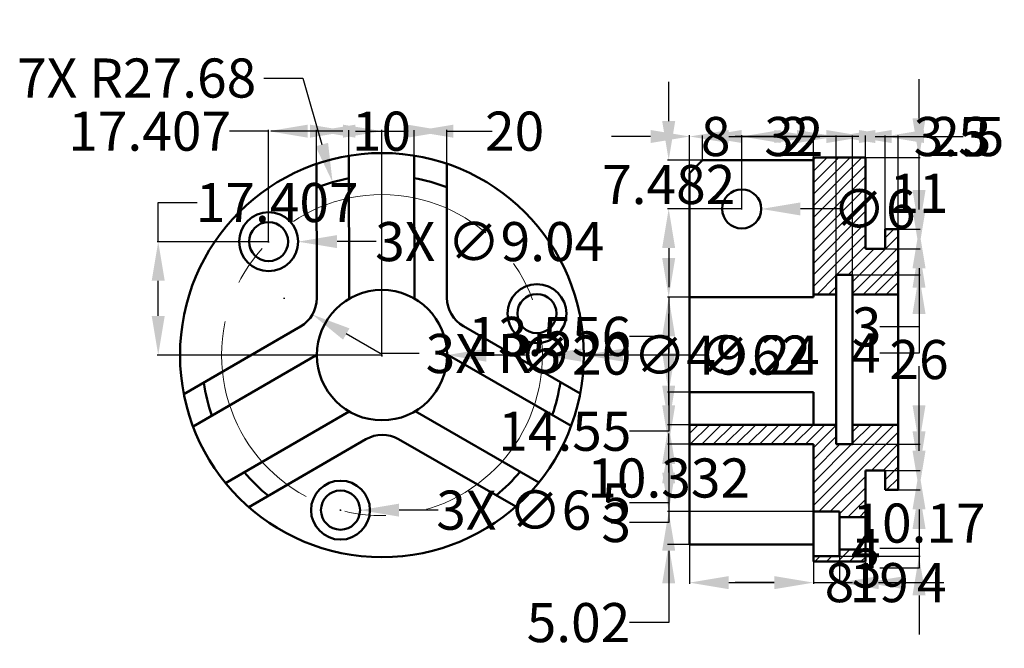
# Model space of a CAD drawing. Units: millimetres. Extents: x 91 to 242, y 23 to 120.
import ezdxf

# ---------------------------------------------------------------- set-up
doc = ezdxf.new("R2010")
doc.units = ezdxf.units.MM
doc.header["$MEASUREMENT"] = 0
doc.linetypes.add('CENTER', pattern=[50.8, 31.75, -6.35, 6.35, -6.35])
for name, color, linetype, lineweight in [('M-CNTR', 4, 'CENTER', 18), ('M-DIMS', 2, 'Continuous', 18), ('M-HATC', 8, 'Continuous', 18), ('M-OUTL', 7, 'Continuous', 50)]:
    doc.layers.add(name, color=color, linetype=linetype, lineweight=lineweight)
doc.styles.get("Standard").update_dxf_attribs({"font": 'arial.ttf'})
doc.dimstyles.get("Standard").update_dxf_attribs({"dimtxt": 6, "dimasz": 6, "dimexe": 0.18, "dimexo": 0.0625, "dimgap": 0.09, "dimtad": 0, "dimtih": 1, "dimtoh": 1, "dimdec": 0, "dimzin": 0, "dimdsep": 46, "dimtxsty": 'Standard', "dimcen": 0.09, "dimadec": 0, "dimazin": 0, "dimtfac": 1, "dimtdec": 0, "dimtofl": 0, "dimtmove": 0, "dimatfit": 3, "dimfxl": 1, "dimtolj": 1, "dimtzin": 0, "dimarcsym": 0})

# ---------------------------------------------------------------- blocks, each defined once
blk = doc.blocks.new('HOLE-CBORE')
for radius in [4.52, 3]:
    blk.add_circle((140.38, 44.32), radius)
blk = doc.blocks.new('*D2')
at = {"layer": 'Defpoints', "color": 0, "transparency": 16777216}
for p in [(151.679954, 102.447071), (141.679978, 98.680142), (151.679954, 98.702087)]:
    blk.add_point(p, dxfattribs=at)
at = {"layer": 'M-DIMS', "color": 0, "lineweight": -2, "transparency": 16777216}
for p, q in [((135.679978, 102.447071), (129.679978, 102.447071)), ((141.679978, 98.742642), (141.679978, 102.627071)), ((151.679954, 98.764587), (151.679954, 102.627071)), ((157.679954, 102.447071), (163.679954, 102.447071))]:
    blk.add_line(p, q, dxfattribs=at)
at = {"layer": 'M-DIMS', "color": 0, "transparency": 16777216}
for points in [[(135.679978, 103.447071), (135.679978, 101.447071), (141.679978, 102.447071)], [(157.679954, 103.447071), (157.679954, 101.447071), (151.679954, 102.447071)]]:
    blk.add_solid(points, dxfattribs=at)
at = {"layer": 'M-DIMS', "color": 0, "transparency": 16777216, "insert": (146.679966, 102.447071), "char_height": 6, "attachment_point": 5}
blk.add_mtext('\\A1;10', dxfattribs=at)
blk = doc.blocks.new('*D3')
at = {"layer": 'Defpoints', "color": 0, "transparency": 16777216}
for p in [(156.68, 102.45), (136.68, 97.42), (156.68, 97.46)]:
    blk.add_point(p, dxfattribs=at)
at = {"layer": 'M-DIMS', "color": 0, "lineweight": -2, "transparency": 16777216}
for p, q in [((136.68, 97.48), (136.68, 102.63)), ((142.68, 102.45), (150.68, 102.45)), ((156.68, 97.52), (156.68, 102.63)), ((156.68, 102.45), (162.68, 102.45))]:
    blk.add_line(p, q, dxfattribs=at)
at = {"layer": 'M-DIMS', "color": 0, "transparency": 16777216}
for points in [[(142.68, 103.45), (142.68, 101.45), (136.68, 102.45)], [(150.68, 103.45), (150.68, 101.45), (156.68, 102.45)]]:
    blk.add_solid(points, dxfattribs=at)
at = {"layer": 'M-DIMS', "color": 0, "transparency": 16777216, "insert": (167.11, 102.45), "char_height": 6, "attachment_point": 5}
blk.add_mtext('\\A1;20', dxfattribs=at)
blk = doc.blocks.new('*D4')
at = {"layer": 'Defpoints', "color": 0, "transparency": 16777216}
for p in [(129.34, 102.45), (129.34, 85.5), (146.75, 68.1)]:
    blk.add_point(p, dxfattribs=at)
at = {"layer": 'M-DIMS', "color": 0, "lineweight": -2, "transparency": 16777216}
for p, q in [((129.34, 102.45), (123.34, 102.45)), ((129.34, 85.57), (129.34, 102.63)), ((140.75, 102.45), (135.34, 102.45)), ((146.75, 68.16), (146.75, 102.63))]:
    blk.add_line(p, q, dxfattribs=at)
at = {"layer": 'M-DIMS', "color": 0, "transparency": 16777216}
for points in [[(135.34, 103.45), (135.34, 101.45), (129.34, 102.45)], [(140.75, 103.45), (140.75, 101.45), (146.75, 102.45)]]:
    blk.add_solid(points, dxfattribs=at)
at = {"layer": 'M-DIMS', "color": 0, "transparency": 16777216, "insert": (111.08, 102.45), "char_height": 6, "attachment_point": 5}
blk.add_mtext('\\A1;17.407', dxfattribs=at)
blk = doc.blocks.new('*D5')
at = {"layer": 'Defpoints', "color": 0, "transparency": 16777216}
for p in [(112.4, 85.5), (129.34, 85.5), (146.75, 68.1)]:
    blk.add_point(p, dxfattribs=at)
at = {"layer": 'M-DIMS', "color": 0, "lineweight": -2, "transparency": 16777216}
for p, q in [((112.4, 85.5), (112.4, 91.5)), ((112.4, 91.5), (118.4, 91.5)), ((129.28, 85.5), (112.22, 85.5)), ((112.4, 74.1), (112.4, 79.5)), ((146.68, 68.1), (112.22, 68.1))]:
    blk.add_line(p, q, dxfattribs=at)
at = {"layer": 'M-DIMS', "color": 0, "transparency": 16777216}
for points in [[(111.4, 79.5), (113.4, 79.5), (112.4, 85.5)], [(111.4, 74.1), (113.4, 74.1), (112.4, 68.1)]]:
    blk.add_solid(points, dxfattribs=at)
at = {"layer": 'M-DIMS', "color": 0, "transparency": 16777216, "insert": (130.66, 91.5), "char_height": 6, "attachment_point": 5}
blk.add_mtext('\\A1;17.407', dxfattribs=at)
blk = doc.blocks.new('*D6')
at = {"layer": 'Defpoints', "color": 0, "transparency": 16777216}
for p in [(225.97, 101.63), (193.97, 96.01), (225.97, 87.42)]:
    blk.add_point(p, dxfattribs=at)
at = {"layer": 'M-DIMS', "color": 0, "lineweight": -2, "transparency": 16777216}
for p, q in [((193.97, 96.07), (193.97, 101.81)), ((199.97, 101.63), (205.62, 101.63)), ((219.97, 101.63), (214.33, 101.63)), ((225.97, 87.48), (225.97, 101.81))]:
    blk.add_line(p, q, dxfattribs=at)
at = {"layer": 'M-DIMS', "color": 0, "transparency": 16777216}
for points in [[(199.97, 102.63), (199.97, 100.63), (193.97, 101.63)], [(219.97, 102.63), (219.97, 100.63), (225.97, 101.63)]]:
    blk.add_solid(points, dxfattribs=at)
at = {"layer": 'M-DIMS', "color": 0, "transparency": 16777216, "insert": (209.97, 101.63), "char_height": 6, "attachment_point": 5}
blk.add_mtext('\\A1;32', dxfattribs=at)
blk = doc.blocks.new('*D7')
at = {"layer": 'Defpoints', "color": 0, "transparency": 16777216}
for p in [(220.974149, 98.417986), (225.974149, 87.417986), (229.189149, 87.417986)]:
    blk.add_point(p, dxfattribs=at)
at = {"layer": 'M-DIMS', "color": 0, "lineweight": -2, "transparency": 16777216}
for p, q in [((229.189149, 104.417986), (229.189149, 110.417986)), ((221.036649, 98.417986), (229.369149, 98.417986)), ((226.036649, 87.417986), (229.369149, 87.417986)), ((229.189149, 81.417986), (229.189149, 75.417986))]:
    blk.add_line(p, q, dxfattribs=at)
at = {"layer": 'M-DIMS', "color": 0, "transparency": 16777216}
for points in [[(228.189149, 104.417986), (230.189149, 104.417986), (229.189149, 98.417986)], [(228.189149, 81.417986), (230.189149, 81.417986), (229.189149, 87.417986)]]:
    blk.add_solid(points, dxfattribs=at)
at = {"layer": 'M-DIMS', "color": 0, "transparency": 16777216, "insert": (229.189149, 92.917986), "char_height": 6, "attachment_point": 5}
blk.add_mtext('\\A1;11', dxfattribs=at)
blk = doc.blocks.new('*D8')
at = {"layer": 'Defpoints', "color": 0, "transparency": 16777216}
for p in [(225.97, 87.42), (223.97, 84.42), (229.19, 84.42)]:
    blk.add_point(p, dxfattribs=at)
at = {"layer": 'M-DIMS', "color": 0, "lineweight": -2, "transparency": 16777216}
for p, q in [((229.19, 93.42), (229.19, 99.42)), ((226.04, 87.42), (229.37, 87.42)), ((224.04, 84.42), (229.37, 84.42)), ((229.19, 78.42), (229.19, 72.42)), ((229.19, 72.42), (223.19, 72.42))]:
    blk.add_line(p, q, dxfattribs=at)
at = {"layer": 'M-DIMS', "color": 0, "transparency": 16777216}
for points in [[(228.19, 93.42), (230.19, 93.42), (229.19, 87.42)], [(228.19, 78.42), (230.19, 78.42), (229.19, 84.42)]]:
    blk.add_solid(points, dxfattribs=at)
at = {"layer": 'M-DIMS', "color": 0, "transparency": 16777216, "insert": (221.13, 72.42), "char_height": 6, "attachment_point": 5}
blk.add_mtext('\\A1;3', dxfattribs=at)
blk = doc.blocks.new('*D9')
at = {"layer": 'Defpoints', "color": 0, "transparency": 16777216}
for p in [(223.97, 84.42), (218.97, 80.42), (229.19, 80.42)]:
    blk.add_point(p, dxfattribs=at)
at = {"layer": 'M-DIMS', "color": 0, "lineweight": -2, "transparency": 16777216}
for p, q in [((229.19, 90.42), (229.19, 96.42)), ((224.04, 84.42), (229.37, 84.42)), ((219.04, 80.42), (229.37, 80.42)), ((229.19, 74.42), (229.19, 68.42)), ((229.19, 68.42), (223.19, 68.42))]:
    blk.add_line(p, q, dxfattribs=at)
at = {"layer": 'M-DIMS', "color": 0, "transparency": 16777216}
for points in [[(228.19, 90.42), (230.19, 90.42), (229.19, 84.42)], [(228.19, 74.42), (230.19, 74.42), (229.19, 80.42)]]:
    blk.add_solid(points, dxfattribs=at)
at = {"layer": 'M-DIMS', "color": 0, "transparency": 16777216, "insert": (221.02, 68.42), "char_height": 6, "attachment_point": 5}
blk.add_mtext('\\A1;4', dxfattribs=at)
blk = doc.blocks.new('*D10')
at = {"layer": 'Defpoints', "color": 0, "transparency": 16777216}
for p in [(218.97, 80.42), (218.97, 54.42), (229.19, 54.42)]:
    blk.add_point(p, dxfattribs=at)
at = {"layer": 'M-DIMS', "color": 0, "lineweight": -2, "transparency": 16777216}
for p, q in [((219.04, 80.42), (229.37, 80.42)), ((229.19, 74.42), (229.19, 70.57)), ((229.19, 60.42), (229.19, 64.26)), ((219.04, 54.42), (229.37, 54.42))]:
    blk.add_line(p, q, dxfattribs=at)
at = {"layer": 'M-DIMS', "color": 0, "transparency": 16777216}
for points in [[(228.19, 74.42), (230.19, 74.42), (229.19, 80.42)], [(228.19, 60.42), (230.19, 60.42), (229.19, 54.42)]]:
    blk.add_solid(points, dxfattribs=at)
at = {"layer": 'M-DIMS', "color": 0, "transparency": 16777216, "insert": (229.19, 67.42), "char_height": 6, "attachment_point": 5}
blk.add_mtext('\\A1;26', dxfattribs=at)
blk = doc.blocks.new('*D11')
at = {"layer": 'Defpoints', "color": 0, "transparency": 16777216}
for p in [(218.97, 54.42), (223.97, 50.42), (229.19, 50.42)]:
    blk.add_point(p, dxfattribs=at)
at = {"layer": 'M-DIMS', "color": 0, "lineweight": -2, "transparency": 16777216}
for p, q in [((229.19, 60.42), (229.19, 66.42)), ((219.04, 54.42), (229.37, 54.42)), ((224.04, 50.42), (229.37, 50.42)), ((229.19, 44.42), (229.19, 38.42)), ((229.19, 38.42), (223.19, 38.42))]:
    blk.add_line(p, q, dxfattribs=at)
at = {"layer": 'M-DIMS', "color": 0, "transparency": 16777216}
for points in [[(228.19, 60.42), (230.19, 60.42), (229.19, 54.42)], [(228.19, 44.42), (230.19, 44.42), (229.19, 50.42)]]:
    blk.add_solid(points, dxfattribs=at)
at = {"layer": 'M-DIMS', "color": 0, "transparency": 16777216, "insert": (221.02, 38.42), "char_height": 6, "attachment_point": 5}
blk.add_mtext('\\A1;4', dxfattribs=at)
blk = doc.blocks.new('*D12')
at = {"layer": 'Defpoints', "color": 0, "transparency": 16777216}
for p in [(223.97, 50.42), (225.97, 47.42), (229.19, 47.42)]:
    blk.add_point(p, dxfattribs=at)
at = {"layer": 'M-DIMS', "color": 0, "lineweight": -2, "transparency": 16777216}
for p, q in [((229.19, 56.42), (229.19, 62.42)), ((224.04, 50.42), (229.37, 50.42)), ((226.04, 47.42), (229.37, 47.42)), ((229.19, 41.42), (229.19, 35.42)), ((229.19, 35.42), (223.19, 35.42))]:
    blk.add_line(p, q, dxfattribs=at)
at = {"layer": 'M-DIMS', "color": 0, "transparency": 16777216}
for points in [[(228.19, 56.42), (230.19, 56.42), (229.19, 50.42)], [(228.19, 41.42), (230.19, 41.42), (229.19, 47.42)]]:
    blk.add_solid(points, dxfattribs=at)
at = {"layer": 'M-DIMS', "color": 0, "transparency": 16777216, "insert": (221.13, 35.42), "char_height": 6, "attachment_point": 5}
blk.add_mtext('\\A1;3', dxfattribs=at)
blk = doc.blocks.new('*D13')
at = {"layer": 'Defpoints', "color": 0, "transparency": 16777216}
for p in [(225.97, 47.42), (216.97, 37.25), (229.19, 37.25)]:
    blk.add_point(p, dxfattribs=at)
at = {"layer": 'M-DIMS', "color": 0, "lineweight": -2, "transparency": 16777216}
for p, q in [((229.19, 53.42), (229.19, 59.42)), ((226.04, 47.42), (229.37, 47.42)), ((217.04, 37.25), (229.37, 37.25)), ((229.19, 31.25), (229.19, 25.25))]:
    blk.add_line(p, q, dxfattribs=at)
at = {"layer": 'M-DIMS', "color": 0, "transparency": 16777216}
for points in [[(228.19, 53.42), (230.19, 53.42), (229.19, 47.42)], [(228.19, 31.25), (230.19, 31.25), (229.19, 37.25)]]:
    blk.add_solid(points, dxfattribs=at)
at = {"layer": 'M-DIMS', "color": 0, "transparency": 16777216, "insert": (229.19, 42.33), "char_height": 6, "attachment_point": 5}
blk.add_mtext('\\A1;10.17', dxfattribs=at)
blk = doc.blocks.new('*D14')
at = {"layer": 'Defpoints', "color": 0, "transparency": 16777216}
for p in [(195.974149, 98.005238), (190.759149, 90.522868), (201.974149, 90.522868)]:
    blk.add_point(p, dxfattribs=at)
at = {"layer": 'M-DIMS', "color": 0, "lineweight": -2, "transparency": 16777216}
for p, q in [((190.759149, 104.005238), (190.759149, 110.005238)), ((195.911649, 98.005238), (190.579149, 98.005238)), ((201.911649, 90.522868), (190.579149, 90.522868)), ((190.759149, 84.522868), (190.759149, 78.522868))]:
    blk.add_line(p, q, dxfattribs=at)
at = {"layer": 'M-DIMS', "color": 0, "transparency": 16777216}
for points in [[(189.759149, 104.005238), (191.759149, 104.005238), (190.759149, 98.005238)], [(189.759149, 84.522868), (191.759149, 84.522868), (190.759149, 90.522868)]]:
    blk.add_solid(points, dxfattribs=at)
at = {"layer": 'M-DIMS', "color": 0, "transparency": 16777216, "insert": (190.759149, 94.264053), "char_height": 6, "attachment_point": 5}
blk.add_mtext('\\A1;7.482', dxfattribs=at)
blk = doc.blocks.new('*D15')
at = {"layer": 'Defpoints', "color": 0, "transparency": 16777216}
for p in [(201.97, 90.52), (190.76, 76.97), (193.97, 76.97)]:
    blk.add_point(p, dxfattribs=at)
at = {"layer": 'M-DIMS', "color": 0, "lineweight": -2, "transparency": 16777216}
for p, q in [((201.91, 90.52), (190.58, 90.52)), ((190.76, 84.52), (190.76, 82.97)), ((193.91, 76.97), (190.58, 76.97)), ((190.76, 76.97), (190.76, 70.97)), ((190.76, 70.97), (184.76, 70.97))]:
    blk.add_line(p, q, dxfattribs=at)
at = {"layer": 'M-DIMS', "color": 0, "transparency": 16777216}
for points in [[(189.76, 84.52), (191.76, 84.52), (190.76, 90.52)], [(189.76, 82.97), (191.76, 82.97), (190.76, 76.97)]]:
    blk.add_solid(points, dxfattribs=at)
at = {"layer": 'M-DIMS', "color": 0, "transparency": 16777216, "insert": (172.5, 70.97), "char_height": 6, "attachment_point": 5}
blk.add_mtext('\\A1;13.556', dxfattribs=at)
blk = doc.blocks.new('*D16')
at = {"layer": 'Defpoints', "color": 0, "transparency": 16777216}
for p in [(193.97, 76.97), (190.76, 62.42), (193.97, 62.42)]:
    blk.add_point(p, dxfattribs=at)
at = {"layer": 'M-DIMS', "color": 0, "lineweight": -2, "transparency": 16777216}
for p, q in [((193.91, 76.97), (190.58, 76.97)), ((190.76, 70.97), (190.76, 68.42)), ((193.91, 62.42), (190.58, 62.42)), ((190.76, 62.42), (190.76, 56.42)), ((190.76, 56.42), (184.76, 56.42))]:
    blk.add_line(p, q, dxfattribs=at)
at = {"layer": 'M-DIMS', "color": 0, "transparency": 16777216}
for points in [[(189.76, 70.97), (191.76, 70.97), (190.76, 76.97)], [(189.76, 68.42), (191.76, 68.42), (190.76, 62.42)]]:
    blk.add_solid(points, dxfattribs=at)
at = {"layer": 'M-DIMS', "color": 0, "transparency": 16777216, "insert": (174.81, 56.42), "char_height": 6, "attachment_point": 5}
blk.add_mtext('\\A1;14.55', dxfattribs=at)
blk = doc.blocks.new('*D17')
at = {"layer": 'Defpoints', "color": 0, "transparency": 16777216}
for p in [(193.97, 62.42), (190.76, 57.42), (193.97, 57.42)]:
    blk.add_point(p, dxfattribs=at)
at = {"layer": 'M-DIMS', "color": 0, "lineweight": -2, "transparency": 16777216}
for p, q in [((190.76, 68.42), (190.76, 74.42)), ((193.91, 62.42), (190.58, 62.42)), ((193.91, 57.42), (190.58, 57.42)), ((190.76, 51.42), (190.76, 45.42)), ((190.76, 45.42), (184.76, 45.42))]:
    blk.add_line(p, q, dxfattribs=at)
at = {"layer": 'M-DIMS', "color": 0, "transparency": 16777216}
for points in [[(189.76, 68.42), (191.76, 68.42), (190.76, 62.42)], [(189.76, 51.42), (191.76, 51.42), (190.76, 57.42)]]:
    blk.add_solid(points, dxfattribs=at)
at = {"layer": 'M-DIMS', "color": 0, "transparency": 16777216, "insert": (182.68, 45.42), "char_height": 6, "attachment_point": 5}
blk.add_mtext('\\A1;5', dxfattribs=at)
blk = doc.blocks.new('*D18')
at = {"layer": 'Defpoints', "color": 0, "transparency": 16777216}
for p in [(193.97, 57.42), (190.76, 54.42), (193.97, 54.42)]:
    blk.add_point(p, dxfattribs=at)
at = {"layer": 'M-DIMS', "color": 0, "lineweight": -2, "transparency": 16777216}
for p, q in [((190.76, 63.42), (190.76, 69.42)), ((193.91, 57.42), (190.58, 57.42)), ((193.91, 54.42), (190.58, 54.42)), ((190.76, 48.42), (190.76, 42.42)), ((190.76, 42.42), (184.76, 42.42))]:
    blk.add_line(p, q, dxfattribs=at)
at = {"layer": 'M-DIMS', "color": 0, "transparency": 16777216}
for points in [[(189.76, 63.42), (191.76, 63.42), (190.76, 57.42)], [(189.76, 48.42), (191.76, 48.42), (190.76, 54.42)]]:
    blk.add_solid(points, dxfattribs=at)
at = {"layer": 'M-DIMS', "color": 0, "transparency": 16777216, "insert": (182.7, 42.42), "char_height": 6, "attachment_point": 5}
blk.add_mtext('\\A1;3', dxfattribs=at)
blk = doc.blocks.new('*D19')
at = {"layer": 'Defpoints', "color": 0, "transparency": 16777216}
for p in [(193.97, 54.42), (190.76, 44.09), (212.97, 44.09)]:
    blk.add_point(p, dxfattribs=at)
at = {"layer": 'M-DIMS', "color": 0, "lineweight": -2, "transparency": 16777216}
for p, q in [((190.76, 60.42), (190.76, 66.42)), ((193.91, 54.42), (190.58, 54.42)), ((212.91, 44.09), (190.58, 44.09)), ((190.76, 38.09), (190.76, 32.09))]:
    blk.add_line(p, q, dxfattribs=at)
at = {"layer": 'M-DIMS', "color": 0, "transparency": 16777216}
for points in [[(189.76, 60.42), (191.76, 60.42), (190.76, 54.42)], [(189.76, 38.09), (191.76, 38.09), (190.76, 44.09)]]:
    blk.add_solid(points, dxfattribs=at)
at = {"layer": 'M-DIMS', "color": 0, "transparency": 16777216, "insert": (190.76, 49.25), "char_height": 6, "attachment_point": 5}
blk.add_mtext('\\A1;10.332', dxfattribs=at)
blk = doc.blocks.new('*D20')
at = {"layer": 'Defpoints', "color": 0, "transparency": 16777216}
for p in [(212.97, 44.09), (190.76, 39.07), (193.97, 39.07)]:
    blk.add_point(p, dxfattribs=at)
at = {"layer": 'M-DIMS', "color": 0, "lineweight": -2, "transparency": 16777216}
for p, q in [((190.76, 50.09), (190.76, 56.09)), ((212.91, 44.09), (190.58, 44.09)), ((193.91, 39.07), (190.58, 39.07)), ((190.76, 33.07), (190.76, 27.07)), ((190.76, 27.07), (184.76, 27.07))]:
    blk.add_line(p, q, dxfattribs=at)
at = {"layer": 'M-DIMS', "color": 0, "transparency": 16777216}
for points in [[(189.76, 50.09), (191.76, 50.09), (190.76, 44.09)], [(189.76, 33.07), (191.76, 33.07), (190.76, 39.07)]]:
    blk.add_solid(points, dxfattribs=at)
at = {"layer": 'M-DIMS', "color": 0, "transparency": 16777216, "insert": (176.91, 27.07), "char_height": 6, "attachment_point": 5}
blk.add_mtext('\\A1;5.02', dxfattribs=at)
blk = doc.blocks.new('*D21')
at = {"layer": 'Defpoints', "color": 0, "transparency": 16777216}
for p in [(193.97, 39.07), (212.97, 39.07), (212.97, 33.2)]:
    blk.add_point(p, dxfattribs=at)
at = {"layer": 'M-DIMS', "color": 0, "lineweight": -2, "transparency": 16777216}
for p, q in [((193.97, 39), (193.97, 33.02)), ((212.97, 39), (212.97, 33.02)), ((199.97, 33.2), (206.97, 33.2)), ((212.97, 33.2), (218.97, 33.2))]:
    blk.add_line(p, q, dxfattribs=at)
at = {"layer": 'M-DIMS', "color": 0, "transparency": 16777216}
for points in [[(199.97, 34.2), (199.97, 32.2), (193.97, 33.2)], [(206.97, 34.2), (206.97, 32.2), (212.97, 33.2)]]:
    blk.add_solid(points, dxfattribs=at)
at = {"layer": 'M-DIMS', "color": 0, "transparency": 16777216, "insert": (223.09, 33.2), "char_height": 6, "attachment_point": 5}
blk.add_mtext('\\A1;19', dxfattribs=at)
blk = doc.blocks.new('*D22')
at = {"layer": 'Defpoints', "color": 0, "transparency": 16777216}
for p in [(212.974149, 36.417986), (220.974149, 36.417986), (220.974149, 33.202986)]:
    blk.add_point(p, dxfattribs=at)
at = {"layer": 'M-DIMS', "color": 0, "lineweight": -2, "transparency": 16777216}
for p, q in [((212.974149, 36.355486), (212.974149, 33.022986)), ((220.974149, 36.355486), (220.974149, 33.022986)), ((206.974149, 33.202986), (200.974149, 33.202986)), ((226.974149, 33.202986), (232.974149, 33.202986))]:
    blk.add_line(p, q, dxfattribs=at)
at = {"layer": 'M-DIMS', "color": 0, "transparency": 16777216}
for points in [[(206.974149, 34.202986), (206.974149, 32.202986), (212.974149, 33.202986)], [(226.974149, 34.202986), (226.974149, 32.202986), (220.974149, 33.202986)]]:
    blk.add_solid(points, dxfattribs=at)
at = {"layer": 'M-DIMS', "color": 0, "transparency": 16777216, "insert": (216.974149, 33.202986), "char_height": 6, "attachment_point": 5}
blk.add_mtext('\\A1;8', dxfattribs=at)
blk = doc.blocks.new('*D23')
at = {"layer": 'Defpoints', "color": 0, "transparency": 16777216}
for p in [(223.97, 101.63), (220.97, 84.42), (223.97, 84.42)]:
    blk.add_point(p, dxfattribs=at)
at = {"layer": 'M-DIMS', "color": 0, "lineweight": -2, "transparency": 16777216}
for p, q in [((214.97, 101.63), (208.97, 101.63)), ((220.97, 84.48), (220.97, 101.81)), ((223.97, 84.48), (223.97, 101.81)), ((229.97, 101.63), (235.97, 101.63))]:
    blk.add_line(p, q, dxfattribs=at)
at = {"layer": 'M-DIMS', "color": 0, "transparency": 16777216}
for points in [[(214.97, 102.63), (214.97, 100.63), (220.97, 101.63)], [(229.97, 102.63), (229.97, 100.63), (223.97, 101.63)]]:
    blk.add_solid(points, dxfattribs=at)
at = {"layer": 'M-DIMS', "color": 0, "transparency": 16777216, "insert": (238.03, 101.63), "char_height": 6, "attachment_point": 5}
blk.add_mtext('\\A1;3', dxfattribs=at)
blk = doc.blocks.new('*D24')
at = {"layer": 'Defpoints', "color": 0, "transparency": 16777216}
for p in [(218.97, 101.63), (216.47, 80.42), (218.97, 80.42)]:
    blk.add_point(p, dxfattribs=at)
at = {"layer": 'M-DIMS', "color": 0, "lineweight": -2, "transparency": 16777216}
for p, q in [((210.47, 101.63), (204.47, 101.63)), ((216.47, 80.48), (216.47, 101.81)), ((218.97, 80.48), (218.97, 101.81)), ((224.97, 101.63), (230.97, 101.63))]:
    blk.add_line(p, q, dxfattribs=at)
at = {"layer": 'M-DIMS', "color": 0, "transparency": 16777216}
for points in [[(210.47, 102.63), (210.47, 100.63), (216.47, 101.63)], [(224.97, 102.63), (224.97, 100.63), (218.97, 101.63)]]:
    blk.add_solid(points, dxfattribs=at)
at = {"layer": 'M-DIMS', "color": 0, "transparency": 16777216, "insert": (236.6, 101.63), "char_height": 6, "attachment_point": 5}
blk.add_mtext('\\A1;2.5', dxfattribs=at)
blk = doc.blocks.new('*D25')
at = {"layer": 'Defpoints', "color": 0, "transparency": 16777216}
for p in [(216.47, 101.63), (216.47, 80.42), (212.97, 77.42)]:
    blk.add_point(p, dxfattribs=at)
at = {"layer": 'M-DIMS', "color": 0, "lineweight": -2, "transparency": 16777216}
for p, q in [((206.97, 101.63), (200.97, 101.63)), ((212.97, 77.48), (212.97, 101.81)), ((216.47, 80.48), (216.47, 101.81)), ((222.47, 101.63), (228.47, 101.63))]:
    blk.add_line(p, q, dxfattribs=at)
at = {"layer": 'M-DIMS', "color": 0, "transparency": 16777216}
for points in [[(206.97, 102.63), (206.97, 100.63), (212.97, 101.63)], [(222.47, 102.63), (222.47, 100.63), (216.47, 101.63)]]:
    blk.add_solid(points, dxfattribs=at)
at = {"layer": 'M-DIMS', "color": 0, "transparency": 16777216, "insert": (234.05, 101.63), "char_height": 6, "attachment_point": 5}
blk.add_mtext('\\A1;3.5', dxfattribs=at)
blk = doc.blocks.new('*D26')
at = {"layer": 'Defpoints', "color": 0, "transparency": 16777216}
for p in [(195.97, 101.63), (195.97, 98.01), (193.97, 96.01)]:
    blk.add_point(p, dxfattribs=at)
at = {"layer": 'M-DIMS', "color": 0, "lineweight": -2, "transparency": 16777216}
for p, q in [((187.97, 101.63), (181.97, 101.63)), ((193.97, 96.07), (193.97, 101.81)), ((195.97, 98.07), (195.97, 101.81)), ((201.97, 101.63), (207.97, 101.63))]:
    blk.add_line(p, q, dxfattribs=at)
at = {"layer": 'M-DIMS', "color": 0, "transparency": 16777216}
for points in [[(187.97, 102.63), (187.97, 100.63), (193.97, 101.63)], [(201.97, 102.63), (201.97, 100.63), (195.97, 101.63)]]:
    blk.add_solid(points, dxfattribs=at)
at = {"layer": 'M-DIMS', "color": 0, "transparency": 16777216, "insert": (210.05, 101.63), "char_height": 6, "attachment_point": 5}
blk.add_mtext('\\A1;2', dxfattribs=at)
blk = doc.blocks.new('*D27')
at = {"layer": 'Defpoints', "color": 0, "transparency": 16777216}
for p in [(201.974149, 101.632986), (193.974149, 96.005238), (201.974149, 90.522868)]:
    blk.add_point(p, dxfattribs=at)
at = {"layer": 'M-DIMS', "color": 0, "lineweight": -2, "transparency": 16777216}
for p, q in [((187.974149, 101.632986), (181.974149, 101.632986)), ((193.974149, 96.067738), (193.974149, 101.812986)), ((201.974149, 90.585368), (201.974149, 101.812986)), ((207.974149, 101.632986), (213.974149, 101.632986))]:
    blk.add_line(p, q, dxfattribs=at)
at = {"layer": 'M-DIMS', "color": 0, "transparency": 16777216}
for points in [[(187.974149, 102.632986), (187.974149, 100.632986), (193.974149, 101.632986)], [(207.974149, 102.632986), (207.974149, 100.632986), (201.974149, 101.632986)]]:
    blk.add_solid(points, dxfattribs=at)
at = {"layer": 'M-DIMS', "color": 0, "transparency": 16777216, "insert": (197.974149, 101.632986), "char_height": 6, "attachment_point": 5}
blk.add_mtext('\\A1;8', dxfattribs=at)
blk = doc.blocks.new('*D28')
at = {"layer": 'Defpoints', "color": 0, "transparency": 16777216}
for p in [(212.97, 44.09), (216.97, 44.09), (216.97, 33.2)]:
    blk.add_point(p, dxfattribs=at)
at = {"layer": 'M-DIMS', "color": 0, "lineweight": -2, "transparency": 16777216}
for p, q in [((212.97, 44.02), (212.97, 33.02)), ((216.97, 44.02), (216.97, 33.02)), ((206.97, 33.2), (200.97, 33.2)), ((222.97, 33.2), (228.97, 33.2))]:
    blk.add_line(p, q, dxfattribs=at)
at = {"layer": 'M-DIMS', "color": 0, "transparency": 16777216}
for points in [[(206.97, 34.2), (206.97, 32.2), (212.97, 33.2)], [(222.97, 34.2), (222.97, 32.2), (216.97, 33.2)]]:
    blk.add_solid(points, dxfattribs=at)
at = {"layer": 'M-DIMS', "color": 0, "transparency": 16777216, "insert": (231.14, 33.2), "char_height": 6, "attachment_point": 5}
blk.add_mtext('\\A1;4', dxfattribs=at)
blk = doc.blocks.new('*D29')
at = {"layer": 'Defpoints', "color": 0, "transparency": 16777216}
for p in [(115.75, 68.1), (177.75, 68.1)]:
    blk.add_point(p, dxfattribs=at)
at = {"layer": 'M-DIMS', "color": 0, "lineweight": -2, "transparency": 16777216}
for p, q in [((146.66, 68.1), (146.84, 68.1)), ((146.75, 68.01), (146.75, 68.19)), ((196.35, 68.1), (183.75, 68.1))]:
    blk.add_line(p, q, dxfattribs=at)
at = {"layer": 'M-DIMS', "color": 0, "transparency": 16777216}
blk.add_solid([(183.75, 69.1), (183.75, 67.1), (177.75, 68.1)], dxfattribs=at)
at = {"layer": 'M-DIMS', "color": 0, "transparency": 16777216, "insert": (203.97, 68.1), "char_height": 6, "attachment_point": 5}
blk.add_mtext('\\A1;∅62', dxfattribs=at)
blk = doc.blocks.new('*D30')
at = {"layer": 'Defpoints', "color": 0, "transparency": 16777216}
for p in [(122.13, 68.1), (171.36, 68.1)]:
    blk.add_point(p, dxfattribs=at)
at = {"layer": 'M-DIMS', "color": 0, "lineweight": -2, "transparency": 16777216}
for p, q in [((146.66, 68.1), (146.84, 68.1)), ((146.75, 68.01), (146.75, 68.19)), ((186.14, 68.1), (177.36, 68.1))]:
    blk.add_line(p, q, dxfattribs=at)
at = {"layer": 'M-DIMS', "color": 0, "transparency": 16777216}
blk.add_solid([(177.36, 69.1), (177.36, 67.1), (171.36, 68.1)], dxfattribs=at)
at = {"layer": 'M-DIMS', "color": 0, "transparency": 16777216, "insert": (199.6, 68.1), "char_height": 6, "attachment_point": 5}
blk.add_mtext('\\A1;∅49.24', dxfattribs=at)
blk = doc.blocks.new('*D31')
at = {"layer": 'Defpoints', "color": 0, "transparency": 16777216}
for p in [(136.75, 68.1), (156.75, 68.1)]:
    blk.add_point(p, dxfattribs=at)
at = {"layer": 'M-DIMS', "color": 0, "lineweight": -2, "transparency": 16777216}
for p, q in [((146.66, 68.1), (146.84, 68.1)), ((146.75, 68.01), (146.75, 68.19)), ((168.75, 68.1), (162.75, 68.1))]:
    blk.add_line(p, q, dxfattribs=at)
at = {"layer": 'M-DIMS', "color": 0, "transparency": 16777216}
blk.add_solid([(162.75, 69.1), (162.75, 67.1), (156.75, 68.1)], dxfattribs=at)
at = {"layer": 'M-DIMS', "color": 0, "transparency": 16777216, "insert": (176.39, 68.1), "char_height": 6, "attachment_point": 5}
blk.add_mtext('\\A1;∅20', dxfattribs=at)
blk = doc.blocks.new('*D32')
at = {"layer": 'Defpoints', "color": 0, "transparency": 16777216}
for p in [(139.16, 94.63), (146.75, 68.01)]:
    blk.add_point(p, dxfattribs=at)
at = {"layer": 'M-DIMS', "color": 0, "lineweight": -2, "transparency": 16777216}
for p, q in [((128.6, 110.6), (134.6, 110.6)), ((134.6, 110.6), (137.51, 100.4)), ((146.75, 67.92), (146.75, 68.1)), ((146.66, 68.01), (146.84, 68.01))]:
    blk.add_line(p, q, dxfattribs=at)
at = {"layer": 'M-DIMS', "color": 0, "transparency": 16777216}
blk.add_solid([(138.47, 100.67), (136.55, 100.12), (139.16, 94.63)], dxfattribs=at)
at = {"layer": 'M-DIMS', "color": 0, "transparency": 16777216, "insert": (109.09, 110.6), "char_height": 6, "attachment_point": 5}
blk.add_mtext('\\A1;7X R27.68', dxfattribs=at)
blk = doc.blocks.new('*D33')
at = {"layer": 'Defpoints', "color": 0, "transparency": 16777216}
for p in [(131.73, 76.81), (136.06, 74.32)]:
    blk.add_point(p, dxfattribs=at)
at = {"layer": 'M-DIMS', "color": 0, "lineweight": -2, "transparency": 16777216}
for p, q in [((131.64, 76.81), (131.82, 76.81)), ((131.73, 76.72), (131.73, 76.9)), ((146.47, 68.35), (141.27, 71.34)), ((152.47, 68.35), (146.47, 68.35))]:
    blk.add_line(p, q, dxfattribs=at)
at = {"layer": 'M-DIMS', "color": 0, "transparency": 16777216}
blk.add_solid([(141.76, 72.2), (140.77, 70.47), (136.06, 74.32)], dxfattribs=at)
at = {"layer": 'M-DIMS', "color": 0, "transparency": 16777216, "insert": (163.86, 68.35), "char_height": 6, "attachment_point": 5}
blk.add_mtext('\\A1;3X R5', dxfattribs=at)
blk = doc.blocks.new('*D34')
at = {"layer": 'Defpoints', "color": 0, "transparency": 16777216}
for p in [(124.82, 85.5), (133.86, 85.5)]:
    blk.add_point(p, dxfattribs=at)
at = {"layer": 'M-DIMS', "color": 0, "lineweight": -2, "transparency": 16777216}
for p, q in [((129.25, 85.5), (129.43, 85.5)), ((129.34, 85.41), (129.34, 85.59)), ((145.86, 85.51), (139.86, 85.51))]:
    blk.add_line(p, q, dxfattribs=at)
at = {"layer": 'M-DIMS', "color": 0, "transparency": 16777216}
blk.add_solid([(139.86, 86.51), (139.86, 84.51), (133.86, 85.5)], dxfattribs=at)
at = {"layer": 'M-DIMS', "color": 0, "transparency": 16777216, "insert": (163.28, 85.51), "char_height": 6, "attachment_point": 5}
blk.add_mtext('\\A1;3X ∅9.04', dxfattribs=at)
blk = doc.blocks.new('*D35')
at = {"layer": 'Defpoints', "color": 0, "transparency": 16777216}
for p in [(137.38, 44.32), (143.38, 44.32)]:
    blk.add_point(p, dxfattribs=at)
at = {"layer": 'M-DIMS', "color": 0, "lineweight": -2, "transparency": 16777216}
for p, q in [((140.29, 44.32), (140.47, 44.32)), ((140.38, 44.23), (140.38, 44.41)), ((155.38, 44.32), (149.38, 44.32))]:
    blk.add_line(p, q, dxfattribs=at)
at = {"layer": 'M-DIMS', "color": 0, "transparency": 16777216}
blk.add_solid([(149.38, 45.32), (149.38, 43.32), (143.38, 44.32)], dxfattribs=at)
at = {"layer": 'M-DIMS', "color": 0, "transparency": 16777216, "insert": (166.98, 44.32), "char_height": 6, "attachment_point": 5}
blk.add_mtext('\\A1;3X ∅6', dxfattribs=at)
blk = doc.blocks.new('*D36')
at = {"layer": 'Defpoints', "color": 0, "transparency": 16777216}
for p in [(198.97, 90.52), (204.97, 90.52)]:
    blk.add_point(p, dxfattribs=at)
at = {"layer": 'M-DIMS', "color": 0, "lineweight": -2, "transparency": 16777216}
for p, q in [((201.88, 90.52), (202.06, 90.52)), ((201.97, 90.43), (201.97, 90.61)), ((216.97, 90.52), (210.97, 90.52))]:
    blk.add_line(p, q, dxfattribs=at)
at = {"layer": 'M-DIMS', "color": 0, "transparency": 16777216}
blk.add_solid([(210.97, 91.52), (210.97, 89.52), (204.97, 90.52)], dxfattribs=at)
at = {"layer": 'M-DIMS', "color": 0, "transparency": 16777216, "insert": (222.29, 90.52), "char_height": 6, "attachment_point": 5}
blk.add_mtext('\\A1;∅6', dxfattribs=at)

msp = doc.modelspace()

# ---------------------------------------------------------------- hatches: boundary and pattern name
at = {"layer": 'M-HATC'}
h = msp.add_hatch(dxfattribs=at)
h.set_pattern_fill('ANSI31', color=256, scale=10)
h.paths.add_polyline_path([(220.9741, 98.418), (212.9741, 98.418), (212.9741, 77.418), (216.4741, 77.418), (216.4741, 80.418), (218.9741, 80.418), (218.9741, 77.418), (225.9741, 77.418), (225.9741, 87.418), (223.9741, 87.418), (223.9741, 84.418), (220.9741, 84.418)])
h.paths.add_polyline_path([(220.9741, 50.418), (223.9741, 50.418), (223.9741, 47.418), (225.9741, 47.418), (225.9741, 57.418), (218.9741, 57.418), (218.9741, 54.418), (216.4741, 54.418), (216.4741, 57.418), (212.9741, 57.418), (193.9741, 57.418), (193.9741, 54.418), (212.9741, 54.418), (212.9741, 44.0863), (216.9741, 44.0863), (216.9741, 43.2588), (220.9741, 43.2588)])
h.paths.add_polyline_path([(220.9741, 38.2588), (216.9741, 38.2588), (216.9741, 37.2477), (212.9741, 37.2477), (212.9741, 36.418), (220.9741, 36.418)])

# ---------------------------------------------------------------- linework, layer by layer
at = {"layer": 'M-CNTR'}
msp.add_circle((146.7471, 68.0971), 24.6179, dxfattribs=at)
at = {"layer": 'M-OUTL'}
for p, q in [((141.7283, 76.7464), (141.68, 98.6801)), ((151.7282, 76.7682), (151.68, 98.7021)), ((220.9741, 98.418), (212.9741, 98.418)), ((212.9741, 76.967), (212.9741, 98.418)), ((220.9741, 84.418), (220.9741, 98.418)), ((136.7281, 76.8253), (136.6827, 97.4179)), ((156.728, 76.8693), (156.6827, 97.4617)), ((195.9741, 98.0052), (193.9741, 96.0052)), ((212.9741, 98.0052), (195.9741, 98.0052)), ((193.9741, 96.0052), (193.9741, 40.0661)), ((225.9741, 87.418), (223.9741, 87.418)), ((223.9741, 84.418), (223.9741, 87.418)), ((225.9741, 87.418), (225.9741, 47.418)), ((223.9741, 84.418), (220.9741, 84.418)), ((216.4741, 54.418), (216.4741, 80.418)), ((218.9741, 80.418), (216.4741, 80.418)), ((218.9741, 54.418), (218.9741, 80.418)), ((218.9741, 67.418), (218.9741, 80.418)), ((216.4741, 77.418), (212.9741, 77.418)), ((225.9741, 77.418), (218.9741, 77.418)), ((225.9741, 67.418), (225.9741, 77.418)), ((212.9741, 76.967), (193.9741, 76.967)), ((134.2376, 72.4897), (116.3328, 62.0997)), ((159.2375, 72.5447), (177.1876, 62.2339)), ((136.7473, 68.1652), (117.7481, 57.1401)), ((156.7465, 68.2094), (175.7942, 57.2681)), ((193.9741, 57.418), (193.9741, 67.418)), ((218.9741, 67.418), (218.9741, 54.418)), ((225.9741, 67.418), (225.9741, 57.418)), ((193.9741, 57.418), (193.9741, 62.418)), ((193.9741, 62.418), (212.9741, 62.418)), ((212.9741, 57.418), (212.9741, 62.418)), ((141.6886, 59.4708), (122.7451, 48.4781)), ((151.8437, 59.4933), (170.8354, 48.5841)), ((212.9741, 57.418), (193.9741, 57.418)), ((216.4741, 57.418), (212.9741, 57.418)), ((225.9741, 57.418), (218.9741, 57.418)), ((144.2757, 55.1912), (126.325, 44.7746)), ((149.2757, 55.2022), (167.2719, 44.8649)), ((212.9741, 54.418), (193.9741, 54.418)), ((212.9741, 36.418), (212.9741, 54.418)), ((218.9741, 54.418), (216.4741, 54.418)), ((220.9741, 36.418), (220.9741, 50.418)), ((223.9741, 50.418), (220.9741, 50.418)), ((223.9741, 47.418), (223.9741, 50.418)), ((225.9741, 47.418), (223.9741, 47.418)), ((216.9741, 44.0863), (212.9741, 44.0863)), ((216.9741, 40.7588), (216.9741, 44.0863)), ((216.9741, 43.2588), (220.9741, 43.2588)), ((220.9741, 43.2588), (220.9741, 40.7588)), ((193.9741, 40.0661), (193.9741, 39.0661)), ((216.9741, 40.7588), (216.9741, 37.2477)), ((220.9741, 40.7588), (220.9741, 38.2588)), ((212.9741, 39.0661), (193.9741, 39.0661)), ((194.9741, 39.0661), (212.9741, 39.0661)), ((212.9741, 37.8634), (212.9741, 36.418)), ((216.9741, 38.2588), (220.9741, 38.2588)), ((216.9741, 37.2477), (212.9741, 37.2477)), ((212.9741, 36.418), (220.9741, 36.418))]:
    msp.add_line(p, q, dxfattribs=at)
for centre, radius in [((146.7471, 68.0971), 31), ((201.9741, 90.5229), 3), ((146.7471, 68.0971), 10)]:
    msp.add_circle(centre, radius, dxfattribs=at)
for centre, radius, start, end in [((146.7471, 68.0071), 27.6816, 100.531464, 111.302257), ((146.7471, 68.0071), 27.6816, 68.948206, 79.719091), ((146.7471, 68.0071), 27.6816, 134.852267, 134.868278), ((131.7281, 76.8143), 5, 300.126111, 0.126111), ((161.728, 76.8803), 5, 180.126111, 240.126111), ((146.7471, 68.0071), 27.6816, 188.6031, 199.39212), ((146.7471, 68.0071), 27.6816, 340.860937, 351.650003), ((146.7852, 50.8666), 5, 60.126111, 120.126111), ((146.7471, 68.0071), 27.6816, 220.204838, 230.957959), ((146.7471, 68.0071), 27.6816, 309.295141, 320.048217)]:
    msp.add_arc(centre, radius, start, end, dxfattribs=at)

# ---------------------------------------------------------------- block references
for p in [(-11.0359, 41.1865), (30.1506, 30.1506), (0, 0)]:
    msp.add_blockref('HOLE-CBORE', p, dxfattribs=at)

# ---------------------------------------------------------------- dimensions: what is measured, and where the dimension line sits
at = {"layer": 'M-DIMS'}
dim = msp.add_radius_dim(center=(146.7471, 68.0071), mpoint=(139.1559, 94.6275), text='7X <>', dimstyle='Standard', override={"dimdec": 2, "dimlfac": 1, "dimrnd": 0, "dimzin": 0, "dimdsep": 46, "dimlunit": 2}, dxfattribs=at)
dim.commit()
dim.dimension.update_dxf_attribs({"geometry": '*D32', "text_midpoint": (109.0889, 110.5997), "dimtype": 164})
for base, p1, p2, override, picture, middle in [((229.1891, 87.418), (220.9741, 98.418), (225.9741, 87.418), {"dimdec": 0, "dimlfac": 1, "dimrnd": 0, "dimzin": 0, "dimdsep": 46, "dimlunit": 2}, '*D7', (229.1891, 92.918)), ((190.7591, 90.5229), (195.9741, 98.0052), (201.9741, 90.5229), {"dimdec": 3, "dimlfac": 1, "dimrnd": 0, "dimzin": 0, "dimdsep": 46, "dimlunit": 2}, '*D14', (190.7591, 94.2641)), ((229.1891, 84.418), (225.9741, 87.418), (223.9741, 84.418), {"dimdec": 0, "dimlfac": 1, "dimrnd": 0, "dimzin": 0, "dimdsep": 46, "dimlunit": 2}, '*D8', (221.1346, 72.418)), ((112.3971, 85.5045), (146.7471, 68.0971), (129.3396, 85.5045), {"dimdec": 3, "dimlfac": 1, "dimrnd": 0, "dimzin": 0, "dimdsep": 46, "dimlunit": 2}, '*D5', (130.659, 91.5045)), ((229.1891, 80.418), (223.9741, 84.418), (218.9741, 80.418), {"dimdec": 0, "dimlfac": 1, "dimrnd": 0, "dimzin": 0, "dimdsep": 46, "dimlunit": 2}, '*D9', (221.0241, 68.418)), ((190.7591, 76.967), (201.9741, 90.5229), (193.9741, 76.967), {"dimdec": 3, "dimlfac": 1, "dimrnd": 0, "dimzin": 0, "dimdsep": 46, "dimlunit": 2}, '*D15', (172.4993, 70.967)), ((229.1891, 54.418), (218.9741, 80.418), (218.9741, 54.418), {"dimdec": 0, "dimlfac": 1, "dimrnd": 0, "dimzin": 0, "dimdsep": 46, "dimlunit": 2}, '*D10', (229.1891, 67.418)), ((190.7591, 62.418), (193.9741, 76.967), (193.9741, 62.418), {"dimdec": 2, "dimlfac": 1, "dimrnd": 0, "dimzin": 0, "dimdsep": 46, "dimlunit": 2}, '*D16', (174.8056, 56.418)), ((190.7591, 57.418), (193.9741, 62.418), (193.9741, 57.418), {"dimdec": 0, "dimlfac": 1, "dimrnd": 0, "dimzin": 0, "dimdsep": 46, "dimlunit": 2}, '*D17', (182.6801, 45.418)), ((190.7591, 54.418), (193.9741, 57.418), (193.9741, 54.418), {"dimdec": 0, "dimlfac": 1, "dimrnd": 0, "dimzin": 0, "dimdsep": 46, "dimlunit": 2}, '*D18', (182.7046, 42.418)), ((190.7591, 44.0863), (193.9741, 54.418), (212.9741, 44.0863), {"dimdec": 3, "dimlfac": 1, "dimrnd": 0, "dimzin": 0, "dimdsep": 46, "dimlunit": 2}, '*D19', (190.7591, 49.2521)), ((229.1891, 50.418), (218.9741, 54.418), (223.9741, 50.418), {"dimdec": 0, "dimlfac": 1, "dimrnd": 0, "dimzin": 0, "dimdsep": 46, "dimlunit": 2}, '*D11', (221.0241, 38.418)), ((229.1891, 47.418), (223.9741, 50.418), (225.9741, 47.418), {"dimdec": 0, "dimlfac": 1, "dimrnd": 0, "dimzin": 0, "dimdsep": 46, "dimlunit": 2}, '*D12', (221.1346, 35.418)), ((229.1891, 37.2477), (225.9741, 47.418), (216.9741, 37.2477), {"dimdec": 2, "dimlfac": 1, "dimrnd": 0, "dimzin": 0, "dimdsep": 46, "dimlunit": 2}, '*D13', (229.1891, 42.3328)), ((190.7591, 39.0661), (212.9741, 44.0863), (193.9741, 39.0661), {"dimdec": 2, "dimlfac": 1, "dimrnd": 0, "dimzin": 0, "dimdsep": 46, "dimlunit": 2}, '*D20', (176.9072, 27.0661))]:
    dim = msp.add_linear_dim(base=base, p1=p1, p2=p2, angle=90, dimstyle='Standard', override=override, dxfattribs=at)
    dim.commit()
    dim.dimension.update_dxf_attribs({"geometry": picture, "text_midpoint": middle})
for base, p1, p2, override, picture, middle in [((129.33963, 102.44707), (146.74711, 68.09707), (129.33963, 85.50454), {"dimdec": 3, "dimlfac": 1, "dimrnd": 0, "dimzin": 0, "dimdsep": 46, "dimlunit": 2}, '*D4', (111.07774, 102.44707)), ((151.68, 102.4471), (141.68, 98.6801), (151.68, 98.7021), {"dimdec": 0, "dimlfac": 1, "dimrnd": 0, "dimzin": 0, "dimdsep": 46, "dimlunit": 2}, '*D2', (146.68, 102.4471)), ((156.6827, 102.4471), (136.6827, 97.4179), (156.6827, 97.4617), {"dimdec": 0, "dimlfac": 1, "dimrnd": 0, "dimzin": 0, "dimdsep": 46, "dimlunit": 2}, '*D3', (167.111, 102.4471)), ((195.9741, 101.633), (193.9741, 96.0052), (195.9741, 98.0052), {"dimdec": 0, "dimlfac": 1, "dimrnd": 0, "dimzin": 0, "dimdsep": 46, "dimlunit": 2}, '*D26', (210.0512, 101.633)), ((201.9741, 101.633), (193.9741, 96.0052), (201.9741, 90.5229), {"dimdec": 0, "dimlfac": 1, "dimrnd": 0, "dimzin": 0, "dimdsep": 46, "dimlunit": 2}, '*D27', (197.9741, 101.633)), ((225.9741, 101.633), (193.9741, 96.0052), (225.9741, 87.418), {"dimdec": 0, "dimlfac": 1, "dimrnd": 0, "dimzin": 0, "dimdsep": 46, "dimlunit": 2}, '*D6', (209.9741, 101.633)), ((216.4741, 101.633), (212.9741, 77.418), (216.4741, 80.418), {"dimdec": 1, "dimlfac": 1, "dimrnd": 0, "dimzin": 0, "dimdsep": 46, "dimlunit": 2}, '*D25', (234.0464, 101.633)), ((218.9741, 101.633), (216.4741, 80.418), (218.9741, 80.418), {"dimdec": 1, "dimlfac": 1, "dimrnd": 0, "dimzin": 0, "dimdsep": 46, "dimlunit": 2}, '*D24', (236.5996, 101.633)), ((223.9741, 101.633), (220.9741, 84.418), (223.9741, 84.418), {"dimdec": 0, "dimlfac": 1, "dimrnd": 0, "dimzin": 0, "dimdsep": 46, "dimlunit": 2}, '*D23', (238.0287, 101.633)), ((216.9741, 33.203), (212.9741, 44.0863), (216.9741, 44.0863), {"dimdec": 0, "dimlfac": 1, "dimrnd": 0, "dimzin": 0, "dimdsep": 46, "dimlunit": 2}, '*D28', (231.1392, 33.203)), ((212.9741, 33.203), (193.9741, 39.0661), (212.9741, 39.0661), {"dimdec": 0, "dimlfac": 1, "dimrnd": 0, "dimzin": 0, "dimdsep": 46, "dimlunit": 2}, '*D21', (223.0853, 33.203)), ((220.9741, 33.203), (212.9741, 36.418), (220.9741, 36.418), {"dimdec": 0, "dimlfac": 1, "dimrnd": 0, "dimzin": 0, "dimdsep": 46, "dimlunit": 2}, '*D22', (216.9741, 33.203))]:
    dim = msp.add_linear_dim(base=base, p1=p1, p2=p2, dimstyle='Standard', override=override, dxfattribs=at)
    dim.commit()
    dim.dimension.update_dxf_attribs({"geometry": picture, "text_midpoint": middle})
for p1, p2, override, picture, middle in [((124.8199, 85.5041), (133.8594, 85.505), {"dimdec": 2, "dimlfac": 1, "dimrnd": 0, "dimzin": 0, "dimdsep": 46, "dimlunit": 2}, '*D34', (145.8594, 85.5062)), ((137.3755, 44.318), (143.3755, 44.318), {"dimdec": 0, "dimlfac": 1, "dimrnd": 0, "dimzin": 0, "dimdsep": 46, "dimlunit": 2}, '*D35', (155.3755, 44.3179))]:
    dim = msp.add_diameter_dim_2p(p1=p1, p2=p2, text='3X <>', dimstyle='Standard', override=override, dxfattribs=at)
    dim.commit()
    dim.dimension.update_dxf_attribs({"geometry": picture, "text_midpoint": middle, "dimtype": 163})
for p1, p2, override, picture, middle in [((198.9741, 90.5227), (204.9741, 90.523), {"dimdec": 0, "dimlfac": 1, "dimrnd": 0, "dimzin": 0, "dimdsep": 46, "dimlunit": 2}, '*D36', (216.9741, 90.5235)), ((115.7471, 68.0971), (177.7471, 68.097), {"dimdec": 0, "dimlfac": 1, "dimrnd": 0, "dimzin": 0, "dimdsep": 46, "dimlunit": 2}, '*D29', (196.3471, 68.097)), ((122.1292, 68.0971), (171.365, 68.097), {"dimdec": 2, "dimlfac": 1, "dimrnd": 0, "dimzin": 0, "dimdsep": 46, "dimlunit": 2}, '*D30', (186.1357, 68.097)), ((136.7471, 68.0971), (156.7471, 68.097), {"dimdec": 0, "dimlfac": 1, "dimrnd": 0, "dimzin": 0, "dimdsep": 46, "dimlunit": 2}, '*D31', (168.7471, 68.0969))]:
    dim = msp.add_diameter_dim_2p(p1=p1, p2=p2, dimstyle='Standard', override=override, dxfattribs=at)
    dim.commit()
    dim.dimension.update_dxf_attribs({"geometry": picture, "text_midpoint": middle, "dimtype": 163})
dim = msp.add_radius_dim(center=(131.7281, 76.8143), mpoint=(136.0639, 74.3241), text='3X <>', dimstyle='Standard', override={"dimdec": 0, "dimlfac": 1, "dimrnd": 0, "dimzin": 0, "dimdsep": 46, "dimlunit": 2}, dxfattribs=at)
dim.commit()
dim.dimension.update_dxf_attribs({"geometry": '*D33', "text_midpoint": (163.8639, 68.3476)})

doc.saveas('drawing.dxf')
